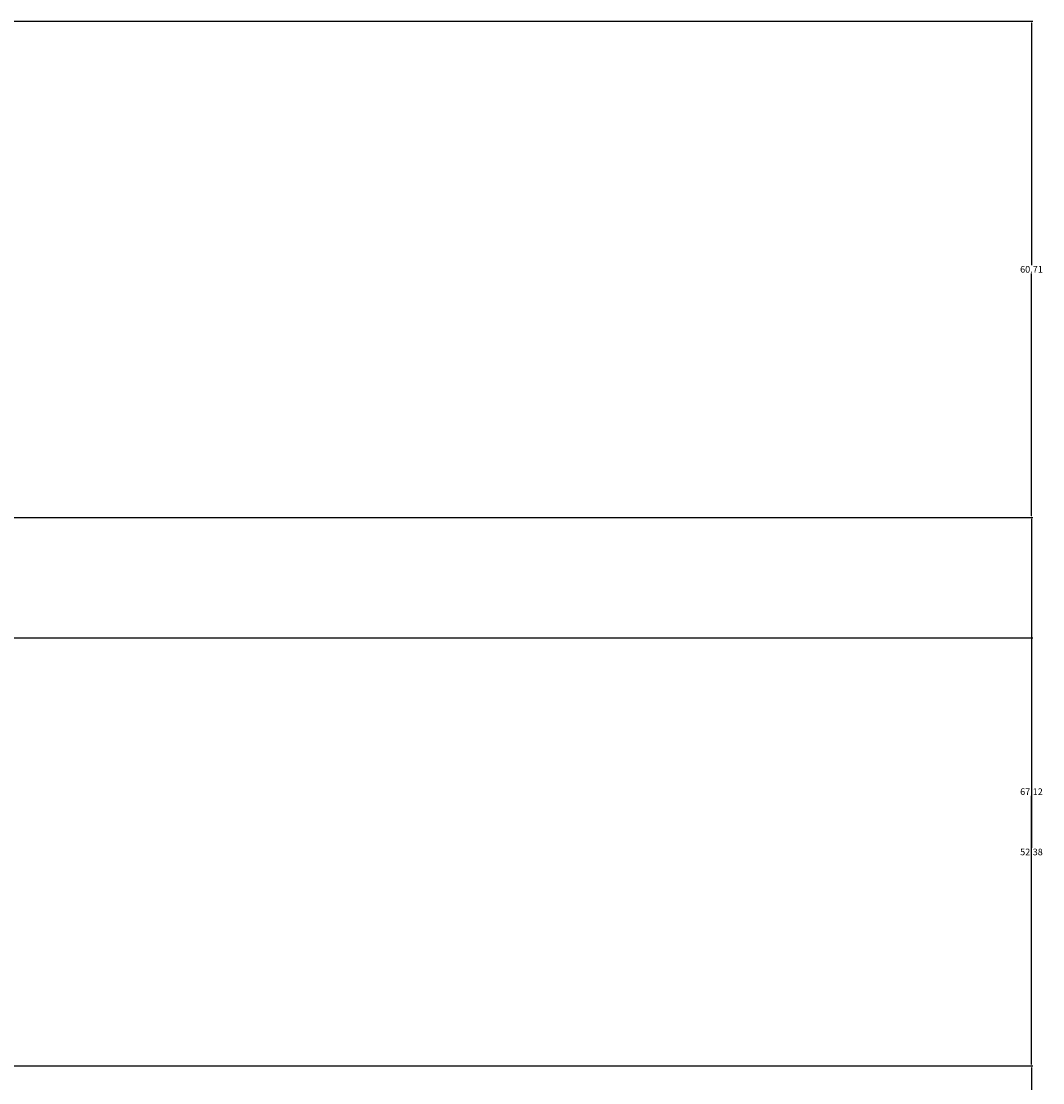
# Model space of a CAD drawing. Units: inches. Extents: x 36 to 594, y 79 to 831.
# Tile 30 of 30: x 469 to 594, y 666 to 796. Entities that reach past the tile are written whole.
import ezdxf

# ---------------------------------------------------------------- set-up
doc = ezdxf.new("R2010")
doc.units = ezdxf.units.IN
doc.header["$MEASUREMENT"] = 0
doc.layers.add('A-ANNO-DIMS', color=2, linetype='Continuous', lineweight=18)
doc.styles.get("Standard").update_dxf_attribs({"font": 'arial.ttf'})
doc.dimstyles.get("Standard").update_dxf_attribs({"dimtxt": 0.8125, "dimasz": 0.18, "dimexe": 0.18, "dimexo": 0.0625, "dimgap": 0.09, "dimtad": 0, "dimtih": 1, "dimtoh": 1, "dimdec": 4, "dimzin": 0, "dimdsep": 46, "dimlunit": 4, "dimtxsty": 'Standard', "dimcen": 0.09, "dimadec": 0, "dimazin": 0, "dimtfac": 1, "dimtdec": 4, "dimtofl": 0, "dimtmove": 0, "dimatfit": 3, "dimfxl": 1, "dimtolj": 1, "dimtzin": 0, "dimarcsym": 0})

# ---------------------------------------------------------------- blocks, each defined once
blk = doc.blocks.new('*D36')
at = {"layer": 'A-ANNO-DIMS', "color": 0, "lineweight": -2, "transparency": 16777216}
for p, q in [((448.452274, 668.212359), (592.848908, 668.212359)), ((592.668908, 668.032359), (592.668908, 631.708609)), ((592.668908, 594.392359), (592.668908, 630.716109)), ((424.55834, 594.212359), (592.848908, 594.212359))]:
    blk.add_line(p, q, dxfattribs=at)
at = {"layer": 'A-ANNO-DIMS', "color": 0, "transparency": 16777216}
for points in [[(592.638908, 668.032359), (592.698908, 668.032359), (592.668908, 668.212359)], [(592.638908, 594.392359), (592.698908, 594.392359), (592.668908, 594.212359)]]:
    blk.add_solid(points, dxfattribs=at)
at = {"layer": 'Defpoints', "color": 0, "transparency": 16777216}
for p in [(448.389774, 668.212359), (592.668908, 668.212359), (424.49584, 594.212359)]:
    blk.add_point(p, dxfattribs=at)
at = {"layer": 'A-ANNO-DIMS', "color": 0, "transparency": 16777216, "insert": (592.668908, 631.212359), "char_height": 0.8125, "attachment_point": 5}
blk.add_mtext('\\A1;74', dxfattribs=at)
blk = doc.blocks.new('*D37')
at = {"layer": 'A-ANNO-DIMS', "color": 0, "lineweight": -2, "transparency": 16777216}
for p, q in [((330.04, 735.34), (592.85, 735.34)), ((592.67, 735.16), (592.67, 702.28)), ((592.67, 668.39), (592.67, 701.27)), ((448.45, 668.21), (592.85, 668.21))]:
    blk.add_line(p, q, dxfattribs=at)
at = {"layer": 'A-ANNO-DIMS', "color": 0, "transparency": 16777216}
for points in [[(592.64, 735.16), (592.7, 735.16), (592.67, 735.34)], [(592.64, 668.39), (592.7, 668.39), (592.67, 668.21)]]:
    blk.add_solid(points, dxfattribs=at)
at = {"layer": 'Defpoints', "color": 0, "transparency": 16777216}
for p in [(329.98, 735.34), (592.67, 735.34), (448.39, 668.21)]:
    blk.add_point(p, dxfattribs=at)
at = {"layer": 'A-ANNO-DIMS', "color": 0, "transparency": 16777216, "insert": (592.67, 701.77), "char_height": 0.812, "attachment_point": 5}
blk.add_mtext('\\A1;67.12', dxfattribs=at)
blk = doc.blocks.new('*D38')
at = {"layer": 'A-ANNO-DIMS', "color": 0, "lineweight": -2, "transparency": 16777216}
for p, q in [((398.15, 796.05), (592.85, 796.05)), ((592.67, 795.87), (592.67, 766.2)), ((592.67, 735.52), (592.67, 765.19)), ((330.04, 735.34), (592.85, 735.34))]:
    blk.add_line(p, q, dxfattribs=at)
at = {"layer": 'A-ANNO-DIMS', "color": 0, "transparency": 16777216}
for points in [[(592.64, 795.87), (592.7, 795.87), (592.67, 796.05)], [(592.64, 735.52), (592.7, 735.52), (592.67, 735.34)]]:
    blk.add_solid(points, dxfattribs=at)
at = {"layer": 'Defpoints', "color": 0, "transparency": 16777216}
for p in [(398.09, 796.05), (592.67, 796.05), (329.98, 735.34)]:
    blk.add_point(p, dxfattribs=at)
at = {"layer": 'A-ANNO-DIMS', "color": 0, "transparency": 16777216, "insert": (592.67, 765.69), "char_height": 0.812, "attachment_point": 5}
blk.add_mtext('\\A1;60.71', dxfattribs=at)
blk = doc.blocks.new('*D41')
at = {"layer": 'A-ANNO-DIMS', "color": 0, "lineweight": -2, "transparency": 16777216}
for p, q in [((341.9, 720.59), (592.85, 720.59)), ((592.67, 720.41), (592.67, 694.91)), ((592.67, 668.39), (592.67, 693.9)), ((448.45, 668.21), (592.85, 668.21))]:
    blk.add_line(p, q, dxfattribs=at)
at = {"layer": 'A-ANNO-DIMS', "color": 0, "transparency": 16777216}
for points in [[(592.64, 720.41), (592.7, 720.41), (592.67, 720.59)], [(592.64, 668.39), (592.7, 668.39), (592.67, 668.21)]]:
    blk.add_solid(points, dxfattribs=at)
at = {"layer": 'Defpoints', "color": 0, "transparency": 16777216}
for p in [(341.84, 720.59), (592.67, 720.59), (448.39, 668.21)]:
    blk.add_point(p, dxfattribs=at)
at = {"layer": 'A-ANNO-DIMS', "color": 0, "transparency": 16777216, "insert": (592.67, 694.4), "char_height": 0.812, "attachment_point": 5}
blk.add_mtext('\\A1;52.38', dxfattribs=at)

msp = doc.modelspace()

# ---------------------------------------------------------------- dimensions: what is measured, and where the dimension line sits
at = {"layer": 'A-ANNO-DIMS'}
for base, p1, p2, override, picture, middle in [((592.6689, 796.0465), (329.982, 735.3373), (398.0873, 796.0465), {"dimdec": 2, "dimlfac": 1, "dimrnd": 0, "dimzin": 0, "dimdsep": 46, "dimlunit": 2}, '*D38', (592.6689, 765.6919)), ((592.6689, 735.3373), (448.3898, 668.2124), (329.982, 735.3373), {"dimdec": 2, "dimlfac": 1, "dimrnd": 0, "dimzin": 0, "dimdsep": 46, "dimlunit": 2}, '*D37', (592.6689, 701.7748)), ((592.6689, 720.595), (448.3898, 668.2124), (341.8367, 720.595), {"dimdec": 2, "dimlfac": 1, "dimrnd": 0, "dimzin": 0, "dimdsep": 46, "dimlunit": 2}, '*D41', (592.6689, 694.4037)), ((592.6689, 668.2124), (424.4958, 594.2124), (448.3898, 668.2124), {"dimdec": 0, "dimlfac": 1, "dimrnd": 0, "dimzin": 0, "dimdsep": 46, "dimlunit": 2}, '*D36', (592.6689, 631.2124))]:
    dim = msp.add_linear_dim(base=base, p1=p1, p2=p2, angle=90, dimstyle='Standard', override=override, dxfattribs=at)
    dim.commit()
    dim.dimension.update_dxf_attribs({"geometry": picture, "text_midpoint": middle})

doc.saveas('drawing.dxf')
